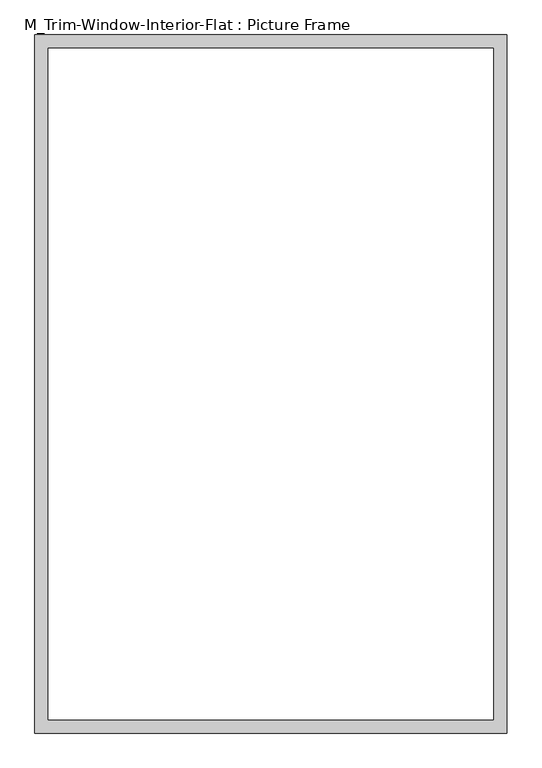
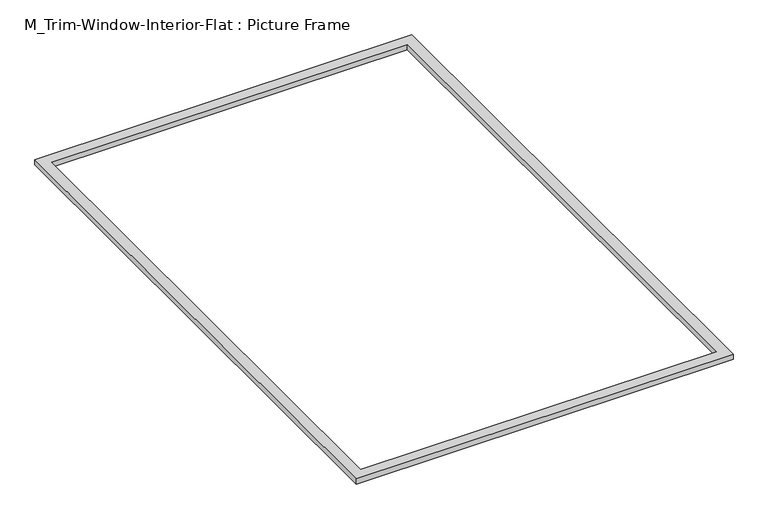
"""IFC4 building model written with IfcOpenShell, lengths in millimetres: proxy geometry, M_Trim-Window-Interior-Flat : Picture Frame."""

from ifc_helpers import new_model, si_unit, origin, origin_with_axes, place, context, project, spatial, polyline, outline, extrude, source, transform, mapped, element, save


def m_trim_window_interior_flat_picture_frame_e5a503a4(model_context):
    return source(origin(), model_context, "Body", "SweptSolid", [
        extrude(outline(polyline([(1047.3, 47.3), (1047.3, -3047.3), (-1047.3, -3047.3), (-1047.3, 47.3), (1047.3, 47.3)]), holes=[polyline([(987.3, -12.7), (-987.3, -12.7), (-987.3, -2987.3), (987.3, -2987.3), (987.3, -12.7)])]), origin_with_axes(), (0.0, 0.0, 1.0), 30.0),
    ])


if __name__ == "__main__":
    model = new_model("IFC4")
    model_context = context("Model", 3, world=origin())
    ifc_project = project(units=[si_unit("LENGTHUNIT", "METRE", prefix="MILLI")], contexts=[model_context])
    site = spatial("IfcSite", under=ifc_project)
    building = spatial("IfcBuilding", under=site)
    placement = place(None, origin())
    m_trim_window_interior_flat_picture_frame_shape = m_trim_window_interior_flat_picture_frame_e5a503a4(model_context)
    element("IfcBuildingElementProxy", 1, Name="M_Trim-Window-Interior-Flat : Picture Frame", ObjectType="M_Trim-Window-Interior-Flat : Picture Frame", at=placement, inside=building, context=model_context, shape_type="MappedRepresentation", body=[
        mapped(m_trim_window_interior_flat_picture_frame_shape, transform((0.0, 0.0, 0.0), x_axis=(1.0, 0.0, 0.0), y_axis=(0.0, 1.0, 0.0), z_axis=(0.0, 0.0, 1.0))),
    ])
    save(model, "model.ifc")

# Revit data of these elements
# Type "M_Trim-Window-Interior-Flat : Picture Frame"
#   Trim Thickness_Picture Frame = 30 mm
#   Trim Width = 60 mm
#   Trim Thickness_with Sill = 20 mm
#   Sill Thickness = 30 mm
#   Opening Width [instance default] = 600 mm
#   Opening Height [instance default] = 900 mm
#   Default Elevation = 1200 mm
#   Sill = no
#   Picture Frame = yes
#   Trim Material [instance default] = none
# Element 1 (IfcBuildingElementProxy, "M_Trim-Window-Interior-Flat : Picture Frame")
#   Opening Width = 2000 mm
#   Opening Height = 3000 mm
#   Trim Material = Wood - Stained
#   Materials on its faces: "Wood - Stained"
# Materials
#   "Wood - Stained": class "Wood", colour RGB 224 178 126, transparency 0, Cost = 0
